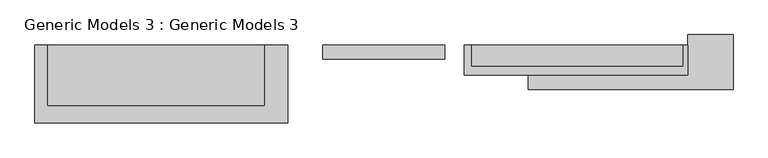
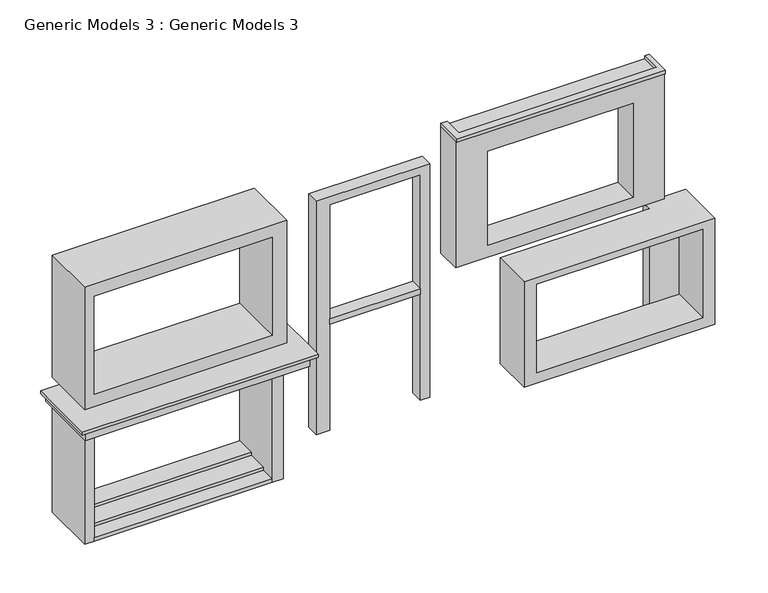
"""IFC4 building model written with IfcOpenShell, lengths in millimetres: proxy geometry, Generic Models 3 : Generic Models 3."""

from ifc_helpers import new_model, si_unit, frame, origin, origin_with_axes, place, context, project, spatial, polyline, outline, extrude, faceted_brep, source, transform, mapped, element, save


def generic_models_3_generic_models_3_c3ffb0d4(model_context):
    return source(origin(), model_context, "Body", "SolidModel", [
        extrude(outline(polyline([(-7792.9097681, -14904.9050846), (-12701.0513104, -14904.9050846), (-12701.0513104, -14246.7339922), (-12548.6513104, -14246.7339922), (-12548.6513104, -14716.9510878), (-7894.5097681, -14716.9510878), (-7894.5097681, -14246.7339922), (-7792.9097681, -14246.7339922), (-7792.9097681, -14904.9050846)])), frame((0.0, 0.0, 6400.8), z_axis=(0.0, 0.0, 1.0), x_axis=(1.0, 0.0, 0.0)), (0.0, 0.0, 1.0), 76.2),
        extrude(outline(polyline([(-13355.5097681, -14551.5339922), (-15489.1097681, -14551.5339922), (-15489.1097681, -14246.7339922), (-13355.5097681, -14246.7339922), (-13355.5097681, -14551.5339922)])), frame((0.0, 0.0, 2636.1562178), z_axis=(0.0, 0.0, 1.0), x_axis=(1.0, 0.0, 0.0)), (0.0, 0.0, 1.0), 139.3776707),
        extrude(outline(polyline([(0.0, -15812.0022226), (0.0, -15489.1097681), (5607.3382011, -15489.1097681), (5607.3382011, -13355.5097681), (0.0, -13355.5097681), (0.0, -13136.1417429), (5810.5382011, -13136.1417429), (5810.5382011, -15812.0022226), (0.0, -15812.0022226)])), frame((0.0, -14551.5339922, 0.0), z_axis=(0.0, 1.0, 0.0), x_axis=(0.0, 0.0, 1.0)), (0.0, 0.0, 1.0), 304.8),
        faceted_brep([(-6801.1895083, -15217.0630685, 2636.1562178), (-11298.1097681, -15217.0630685, 2636.1562178), (-11298.1097681, -15217.0630685, 0.0), (-6801.1895083, -15217.0630685, 0.0), (-7085.3421661, -15217.0630685, 2463.7993261), (-7085.3421661, -15217.0630685, 261.4947537), (-10993.3097681, -15217.0630685, 261.4947537), (-10993.3097681, -15217.0630685, 2463.7993261), (-11298.1097681, -14246.7339922, 0.0), (-11298.1097681, -14246.7339922, 2636.1562178), (-7792.9097681, -14246.7339922, 2636.1562178), (-7792.9097681, -14246.7339922, 2463.7993261), (-10993.3097681, -14246.7339922, 2463.7993261), (-10993.3097681, -14246.7339922, 261.4947537), (-7792.9097681, -14246.7339922, 261.4947537), (-7792.9097681, -14246.7339922, 0.0), (-7792.9097681, -14018.1339922, 0.0), (-6801.1895083, -14018.1339922, 0.0), (-6801.1895083, -14018.1339922, 2636.1562178), (-7792.9097681, -14018.1339922, 2636.1562178), (-7085.3421661, -14246.7339922, 2463.7993261), (-7085.3421661, -14246.7339922, 261.4947537)], [[[0, 1, 2, 3], [4, 5, 6, 7]], [[8, 9, 10, 11, 12, 13, 14, 15]], [[8, 2, 1, 9]], [[2, 8, 15, 16, 17, 3]], [[12, 7, 6, 13]], [[0, 3, 17, 18]], [[1, 0, 18, 19, 10, 9]], [[7, 12, 11, 20, 4]], [[5, 4, 20, 21]], [[6, 5, 21, 14, 13]], [[11, 14, 21, 20]], [[18, 17, 16, 19]], [[19, 16, 15, 14, 11, 10]]]),
        extrude(outline(polyline([(6400.8, -7792.9097681), (6400.8, -12701.0513104), (3246.625042, -12701.0513104), (3246.625042, -7792.9097681), (6400.8, -7792.9097681)]), holes=[polyline([(5884.5037989, -8520.8131537), (3545.3936989, -8520.8131537), (3545.3936989, -11939.1427367), (5884.5037989, -11939.1427367), (5884.5037989, -8520.8131537)])]), frame((0.0, -14856.3339922, 0.0), z_axis=(0.0, 1.0, 0.0), x_axis=(0.0, 0.0, 1.0)), (0.0, 0.0, 1.0), 609.6),
        extrude(outline(polyline([(6400.8, -17091.7535275), (6400.8, -21851.8097681), (3352.8, -21851.8097681), (3352.8, -17091.7535275), (6400.8, -17091.7535275)]), holes=[polyline([(6096.0, -21623.2097681), (6096.0, -17432.2097681), (3659.0308004, -17432.2097681), (3659.0308004, -21623.2097681), (6096.0, -21623.2097681)])]), frame((0.0, -15570.9591665, 0.0), z_axis=(0.0, 1.0, 0.0), x_axis=(0.0, 0.0, 1.0)), (0.0, 0.0, 1.0), 1324.2251742),
        extrude(outline(polyline([(-16577.4286198, -14246.7339922), (-16577.4286198, -15957.6488787), (-22128.6024458, -15957.6488787), (-22128.6024458, -14246.7339922), (-16577.4286198, -14246.7339922)])), frame((0.0, 0.0, 3048.0), z_axis=(0.0, 0.0, 1.0), x_axis=(1.0, 0.0, 0.0)), (0.0, 0.0, 1.0), 76.2),
        extrude(outline(polyline([(-16718.4024458, -15852.6026105), (-22004.2097681, -15852.6026105), (-22004.2097681, -14246.7339922), (-16718.4024458, -14246.7339922), (-16718.4024458, -15852.6026105)])), frame((0.0, 0.0, 2808.8134726), z_axis=(0.0, 0.0, 1.0), x_axis=(1.0, 0.0, 0.0)), (0.0, 0.0, 1.0), 239.1865274),
        extrude(outline(polyline([(-21851.8097681, -15567.5339922), (-21851.8097681, -14246.7339922), (-21623.2097681, -14246.7339922), (-21623.2097681, -15567.5339922), (-21851.8097681, -15567.5339922)])), origin_with_axes(), (0.0, 0.0, 1.0), 2808.8134726),
        extrude(outline(polyline([(-17177.0689588, -14246.7339922), (-17177.0689588, -15570.9591665), (-17432.2097681, -15570.9591665), (-17432.2097681, -14246.7339922), (-17177.0689588, -14246.7339922)])), origin_with_axes(), (0.0, 0.0, 1.0), 2808.8134726),
        extrude(outline(polyline([(-17432.2097681, -15571.0279091), (-21623.2097681, -15571.0279091), (-21623.2097681, -15217.0630685), (-17432.2097681, -15217.0630685), (-17432.2097681, -15571.0279091)])), origin_with_axes(), (0.0, 0.0, 1.0), 84.0916499),
        extrude(outline(polyline([(-17432.2097681, -15217.0630685), (-21623.2097681, -15217.0630685), (-21623.2097681, -14719.1013202), (-17432.2097681, -14719.1013202), (-17432.2097681, -15217.0630685)])), origin_with_axes(), (0.0, 0.0, 1.0), 154.1907953),
        extrude(outline(polyline([(-17432.2097681, -14719.1013202), (-21623.2097681, -14719.1013202), (-21623.2097681, -14246.7339922), (-17432.2097681, -14246.7339922), (-17432.2097681, -14719.1013202)])), origin_with_axes(), (0.0, 0.0, 1.0), 227.670504),
    ])


if __name__ == "__main__":
    model = new_model("IFC4")
    model_context = context("Model", 3, world=origin())
    ifc_project = project(units=[si_unit("LENGTHUNIT", "METRE", prefix="MILLI")], contexts=[model_context])
    site = spatial("IfcSite", under=ifc_project)
    building = spatial("IfcBuilding", under=site)
    placement = place(None, origin())
    generic_models_3_generic_models_3_shape = generic_models_3_generic_models_3_c3ffb0d4(model_context)
    element("IfcBuildingElementProxy", 1, Name="Generic Models 3 : Generic Models 3", ObjectType="Generic Models 3 : Generic Models 3", at=placement, inside=building, context=model_context, shape_type="MappedRepresentation", body=[
        mapped(generic_models_3_generic_models_3_shape, transform((0.0, 0.0, 0.0), x_axis=(1.0, 0.0, 0.0), y_axis=(0.0, 1.0, 0.0), z_axis=(0.0, 0.0, 1.0))),
    ])
    save(model, "model.ifc")
